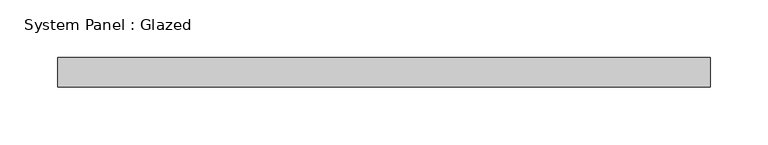
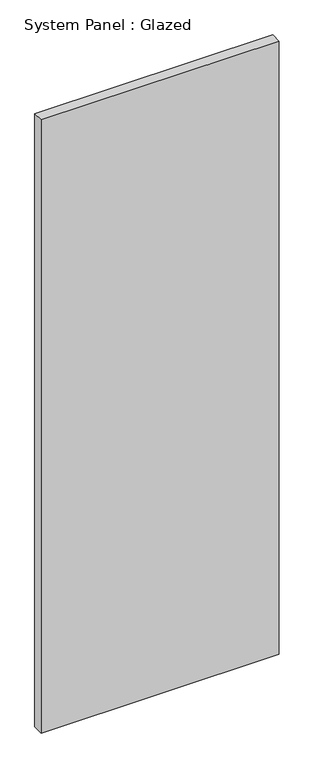
"""IFC4 building model written with IfcOpenShell, lengths in millimetres: plate geometry, System Panel : Glazed."""

from ifc_helpers import new_model, si_unit, origin, origin_with_axes, place, context, project, spatial, polyline, outline, extrude, source, transform, mapped, element, save


def system_panel_glazed_dfff3d37(model_context):
    return source(origin(), model_context, "Body", "SweptSolid", [
        extrude(outline(polyline([(282.575, 19.05), (-282.575, 19.05), (-282.575, 44.45), (282.575, 44.45), (282.575, 19.05)])), origin_with_axes(), (0.0, 0.0, 1.0), 1536.8745067),
    ])


if __name__ == "__main__":
    model = new_model("IFC4")
    model_context = context("Model", 3, world=origin())
    ifc_project = project(units=[si_unit("LENGTHUNIT", "METRE", prefix="MILLI")], contexts=[model_context])
    site = spatial("IfcSite", under=ifc_project)
    building = spatial("IfcBuilding", under=site)
    placement = place(None, origin())
    system_panel_glazed_shape = system_panel_glazed_dfff3d37(model_context)
    element("IfcPlate", 1, ObjectType="System Panel : Glazed", at=placement, inside=building, context=model_context, shape_type="MappedRepresentation", body=[
        mapped(system_panel_glazed_shape, transform((0.0, 0.0, 0.0), x_axis=(1.0, 0.0, 0.0), y_axis=(0.0, 1.0, 0.0), z_axis=(0.0, 0.0, 1.0))),
    ])
    save(model, "model.ifc")

# Revit data of these elements
# Type "System Panel : Glazed"
#   Construction Type Id = "GSP4R"
#   Analytic Construction = "1/8 in Pilkington single glazing"
#   Visual Light Transmittance = 0.9
#   Solar Heat Gain Coefficient = 0.86
#   Heat Transfer Coefficient (U) = 1.18115 BTU/(h·ft²·°F)
#   Define Thermal Properties by = 1
# Element 1 (IfcPlate, "System Panel : Glazed")
#   Materials on its faces: "Glass"
# Materials
#   "Glass": class "Glass", colour RGB 0 128 192, transparency 0.75, Description = "Soda Lime Glass", Cost = 0
